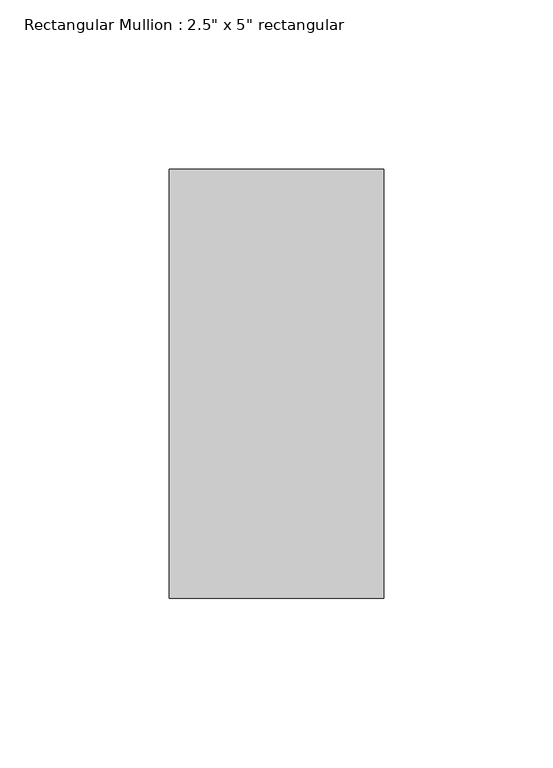
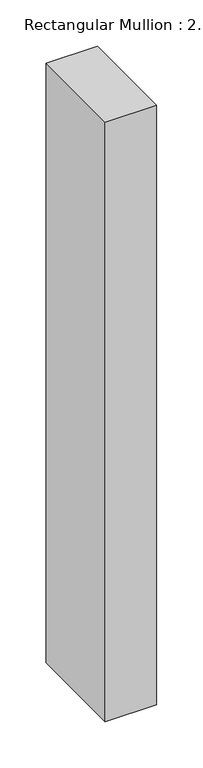
"""IFC4 building model written with IfcOpenShell, lengths in millimetres: member geometry."""

from ifc_helpers import new_model, si_unit, frame, origin, place, context, project, spatial, polyline, outline, extrude, source, transform, mapped, element, save


def member_429f6687(model_context):
    return source(origin(), model_context, "Body", "SweptSolid", [
        extrude(outline(polyline([(0.0, 63.5), (0.0, -63.5), (-63.5, -63.5), (-63.5, 63.5), (0.0, 63.5)])), frame((0.0, 0.0, -787.4), z_axis=(0.0, 0.0, 1.0), x_axis=(1.0, 0.0, 0.0)), (0.0, 0.0, 1.0), 787.4),
    ])


if __name__ == "__main__":
    model = new_model("IFC4")
    model_context = context("Model", 3, world=origin())
    ifc_project = project(units=[si_unit("LENGTHUNIT", "METRE", prefix="MILLI")], contexts=[model_context])
    site = spatial("IfcSite", under=ifc_project)
    building = spatial("IfcBuilding", under=site)
    placement = place(None, origin())
    member_shape = member_429f6687(model_context)
    element("IfcMember", 1, ObjectType="Rectangular Mullion : 2.5\" x 5\" rectangular", at=placement, inside=building, context=model_context, shape_type="MappedRepresentation", body=[
        mapped(member_shape, transform((0.0, 0.0, 0.0), x_axis=(1.0, 0.0, 0.0), y_axis=(0.0, 1.0, 0.0), z_axis=(0.0, 0.0, 1.0))),
    ])
    save(model, "model.ifc")

# Revit data of these elements
# Type "Rectangular Mullion : 2.5\" x 5\" rectangular"
#   built-in parameter 1007304 = 0.416667 (stored number, unit not read)
#   built-in parameter 1007301 = 0.104167 (stored number, unit not read)
#   built-in parameter 1007300 = 0.104167 (stored number, unit not read)
# Element 1 (IfcMember, "Rectangular Mullion : 2.5\" x 5\" rectangular")
#   Materials on its faces: "Iron, Ductile"
# Materials
#   "Iron, Ductile": class "Metal", colour RGB 0 0 0, transparency 0, Description = "Ductile cast iron", Cost = 0
